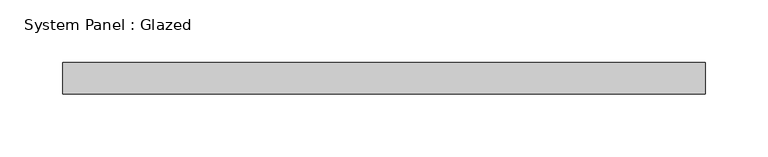
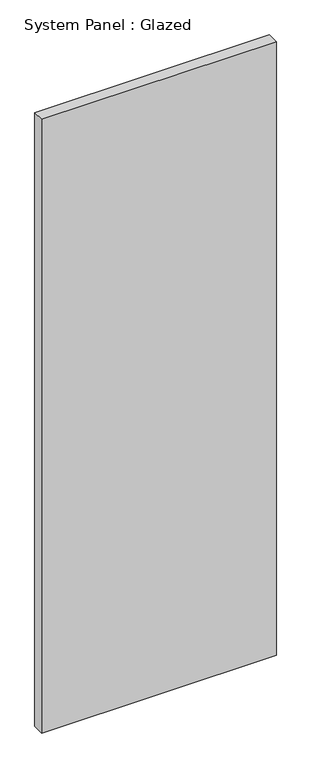
"""IFC4 building model written with IfcOpenShell, lengths in millimetres: plate geometry, System Panel : Glazed."""

from ifc_helpers import new_model, si_unit, origin, origin_with_axes, place, context, project, spatial, polyline, outline, extrude, source, transform, mapped, element, save


def system_panel_glazed_cb7cf9ed(model_context):
    return source(origin(), model_context, "Body", "SweptSolid", [
        extrude(outline(polyline([(257.175, 19.05), (-257.175, 19.05), (-257.175, 44.45), (257.175, 44.45), (257.175, 19.05)])), origin_with_axes(), (0.0, 0.0, 1.0), 1420.2824814),
    ])


if __name__ == "__main__":
    model = new_model("IFC4")
    model_context = context("Model", 3, world=origin())
    ifc_project = project(units=[si_unit("LENGTHUNIT", "METRE", prefix="MILLI")], contexts=[model_context])
    site = spatial("IfcSite", under=ifc_project)
    building = spatial("IfcBuilding", under=site)
    placement = place(None, origin())
    system_panel_glazed_shape = system_panel_glazed_cb7cf9ed(model_context)
    element("IfcPlate", 1, ObjectType="System Panel : Glazed", at=placement, inside=building, context=model_context, shape_type="MappedRepresentation", body=[
        mapped(system_panel_glazed_shape, transform((0.0, 0.0, 0.0), x_axis=(1.0, 0.0, 0.0), y_axis=(0.0, 1.0, 0.0), z_axis=(0.0, 0.0, 1.0))),
    ])
    save(model, "model.ifc")

# Revit data of these elements
# Type "System Panel : Glazed"
#   Construction Type Id = "GSP4R"
#   Analytic Construction = "1/8 in Pilkington single glazing"
#   Visual Light Transmittance = 0.9
#   Solar Heat Gain Coefficient = 0.86
#   Heat Transfer Coefficient (U) = 1.18115 BTU/(h·ft²·°F)
#   Define Thermal Properties by = 1
# Element 1 (IfcPlate, "System Panel : Glazed")
#   Materials on its faces: "Glass"
# Materials
#   "Glass": class "Glass", colour RGB 0 128 192, transparency 0.75, Description = "Soda Lime Glass", Cost = 0
